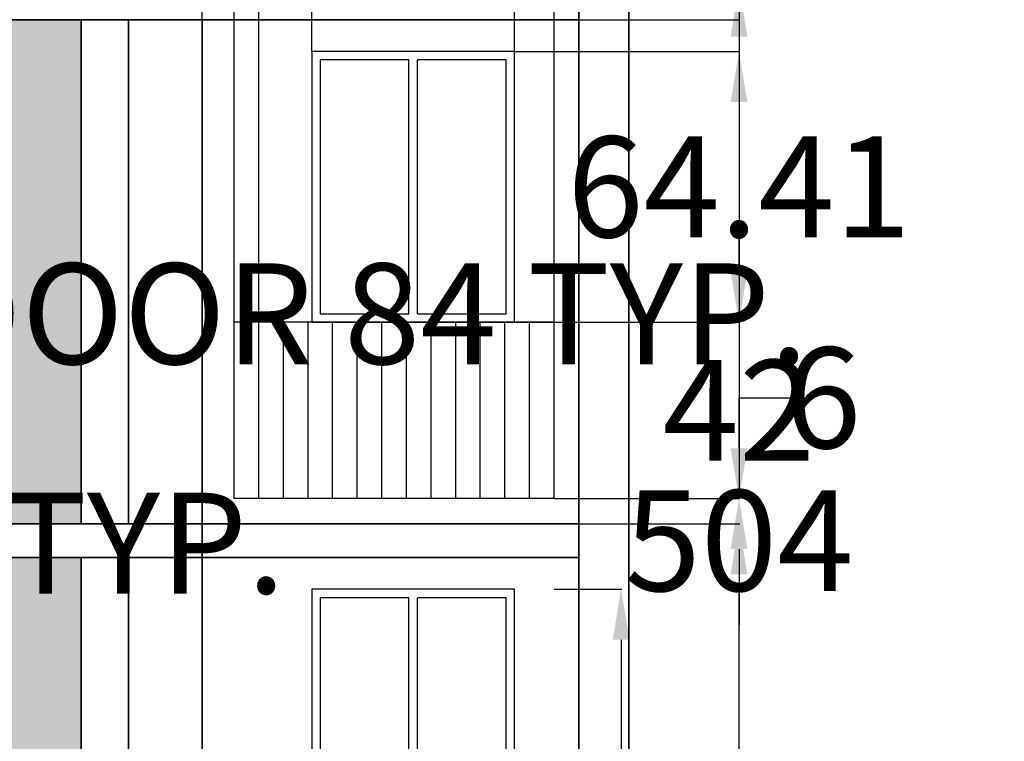
# Model space of a CAD drawing. Units: inches. Extents: x 172 to 828, y 190 to 777.
# Tile 5 of 9: x 474 to 708, y 436 to 607. Entities that reach past the tile are written whole.
import ezdxf

# ---------------------------------------------------------------- set-up
doc = ezdxf.new("R2010")
doc.units = ezdxf.units.IN
doc.header["$MEASUREMENT"] = 0
for name, color, linetype, lineweight in [('A-ANNO-DIMS', 2, 'Continuous', 18), ('A-ELEV', 7, 'Continuous', 35), ('A-ELEV-PATT', 8, 'Continuous', 13), ('A-GLAZ', 3, 'Continuous', 25)]:
    doc.layers.add(name, color=color, linetype=linetype, lineweight=lineweight)
doc.styles.get("Standard").update_dxf_attribs({"font": 'arial.ttf'})
doc.dimstyles.get("Standard").update_dxf_attribs({"dimtxt": 24, "dimasz": 12, "dimexe": 0.18, "dimexo": 0.0625, "dimgap": 0.09, "dimtad": 0, "dimtih": 1, "dimtoh": 1, "dimdec": 0, "dimzin": 0, "dimdsep": 46, "dimlunit": 3, "dimtxsty": 'Standard', "dimcen": 0.09, "dimadec": 0, "dimazin": 0, "dimtfac": 1, "dimtdec": 0, "dimtofl": 0, "dimtmove": 0, "dimatfit": 3, "dimfxl": 1, "dimtolj": 1, "dimtzin": 0, "dimarcsym": 0})
pattern_1 = [(228.012788, (0.72, 1), (-8, -9), [0.134536, -13.319088]), (184.969741, (0.63, 0.9), (12, 1), [0.230868, -22.8559248]), (132.510447, (0.4, 0.88), (10, -11), [0.162788, -16.1160326]), (267.273689, (0.01, 0.63), (1, 20), [0.210238, -20.813558]), (292.833654, (0, 0.42), (-5, 12), [0.206155, -20.4093731]), (357.273689, (0.08, 0.23), (-20, 1), [0.210238, -20.813558]), (37.6942405, (0.29, 0.22), (-13, -10), [0.278029, -27.5248485]), (72.2553284, (0.51, 0.39), (7, 22), [0.262488, -25.9863215]), (121.4295656, (0.59, 0.64), (-8, 13), [0.21095, -20.8840731]), (175.236358, (0.48, 0.82), (11, -1), [0.240832, -11.8007626]), (222.397438, (0.24, 0.84), (-12, -11), [0.311448, -30.833375]), (138.814075, (1, 0.62), (-7, 6), [0.106301, -10.5238448]), (171.4692344, (0.92, 0.69), (13, -2), [0.202237, -20.0215114]), (225, (0.72, 0.72), (-1e-16, -1), [0.141421, -1.2727926]), (203.19859, (0.65, 0.84), (5, 2), [0.076158, -7.5396151]), (291.80141, (0.58, 0.81), (-1, 3), [0.107703, -5.2774618]), (30.963757, (0.62, 0.71), (3, 2), [0.174929, -5.6560229]), (161.56505, (0.77, 0.8), (2, -1), [0.126491, -3.0357867]), (16.38954, (0, 0.81), (10, 3), [0.1772, -17.5428451]), (70.346176, (0.17, 0.86), (-4, -11), [0.148661, -14.7174077]), (293.19859, (0.77, 1), (-2, 5), [0.152315, -7.4634581]), (343.61046, (0.83, 0.86), (-10, 3), [0.1772, -17.5428451]), (339.443955, (0, 0.19), (-5, 2), [0.17088, -8.3731237]), (294.775141, (0.16, 0.13), (-5, 11), [0.143178, -14.1746431]), (66.80141, (0.78, 0), (2, 5), [0.152315, -7.4634581]), (17.354025, (0.84, 0.14), (-13, -4), [0.167631, -16.5954236]), (69.443955, (0.29, 0), (-2, -5), [0.08544, -8.4585637]), (101.309932, (0.72, 0), (-1, 4), [0.05099, -5.0480295]), (165.963757, (0.71, 0.05), (3, -1), [0.206155, -3.9169506]), (186.009006, (0.51, 0.1), (10, 1), [0.19105, -18.9139232]), (303.690068, (0.62, 0.62), (-1, 2), [0.144222, -3.4613293]), (353.1572266, (0.7, 0.5), (17, -2), [0.251794, -24.9275626]), (60.945396, (0.95, 0.47), (-4, -7), [0.102956, -10.1926741]), (90, (1, 0.56), (-1, 1), [0.06, -0.94]), (120.256437, (0.49, 0.13), (4, -7), [0.138924, -13.75352]), (48.012788, (0.42, 0.25), (8, 9), [0.269072, -13.184552]), (0, (0.6, 0.45), (1, 1), [0.26, -0.74]), (325.3048465, (0.86, 0.45), (10, -7), [0.158114, -15.6532743]), (254.054604, (0.99, 0.36), (-1, -4), [0.145602, -7.1345079]), (207.6459754, (0.95, 0.22), (-19, -10), [0.237065, -23.4694742]), (175.426079, (0.74, 0.11), (-13, 1), [0.250799, -24.8290734])]

# ---------------------------------------------------------------- blocks, each defined once
blk = doc.blocks.new('WIN-BALCONY')
for p, q in [((41.59, 44), (41.59, 104.41)), ((43.59, 44), (43.59, 104.41)), ((76.13, 42), (0, 42)), ((0, 0), (0, 42)), ((5.86, 0), (5.86, 42)), ((11.71, 0), (11.71, 42)), ((17.57, 0), (17.57, 42)), ((23.43, 0), (23.43, 42)), ((29.28, 0), (29.28, 42)), ((35.14, 0), (35.14, 42)), ((40.99, 0), (40.99, 42)), ((46.85, 0), (46.85, 42)), ((52.71, 0), (52.71, 42)), ((58.56, 0), (58.56, 42)), ((64.42, 0), (64.42, 42)), ((70.28, 0), (70.28, 42)), ((76.13, 0), (76.13, 42)), ((76.13, 0), (0, 0))]:
    blk.add_line(p, q)
blk.add_lwpolyline([(18.47, 42), (66.72, 42), (66.72, 106.41), (18.47, 106.41)], close=True)
for points in [[(41.59, 104.41), (20.47, 104.41), (20.47, 44), (41.59, 44)], [(43.59, 44), (64.72, 44), (64.72, 104.41), (43.59, 104.41)]]:
    blk.add_lwpolyline(points)
blk = doc.blocks.new('*D4')
at = {"layer": 'A-ANNO-DIMS', "color": 0, "lineweight": -2, "transparency": 16777216}
for p, q in [((601.02, 471.8), (617.1, 471.8)), ((616.92, 459.8), (616.92, 431.1)), ((616.92, 377.39), (616.92, 406.09)), ((601.02, 365.39), (617.1, 365.39))]:
    blk.add_line(p, q, dxfattribs=at)
at = {"layer": 'A-ANNO-DIMS', "color": 0, "transparency": 16777216}
for points in [[(614.92, 459.8), (618.92, 459.8), (616.92, 471.8)], [(614.92, 377.39), (618.92, 377.39), (616.92, 365.39)]]:
    blk.add_solid(points, dxfattribs=at)
at = {"layer": 'Defpoints', "color": 0, "transparency": 16777216}
for p in [(600.96, 471.8), (616.92, 471.8), (600.96, 365.39)]:
    blk.add_point(p, dxfattribs=at)
at = {"layer": 'A-ANNO-DIMS', "color": 0, "transparency": 16777216, "insert": (616.92, 418.6), "char_height": 24, "attachment_point": 5}
blk.add_mtext('\\A1;BALCONY WINDOW 106 TYP.', dxfattribs=at)
blk = doc.blocks.new('*D6')
at = {"layer": 'A-ANNO-DIMS', "color": 0, "lineweight": -2, "transparency": 16777216}
for p, q in [((411.3, 579.39), (424.02, 579.39)), ((423.84, 567.39), (423.84, 549.9)), ((423.84, 507.39), (423.84, 524.88)), ((411.3, 495.39), (424.02, 495.39))]:
    blk.add_line(p, q, dxfattribs=at)
at = {"layer": 'A-ANNO-DIMS', "color": 0, "transparency": 16777216}
for points in [[(421.84, 567.39), (425.84, 567.39), (423.84, 579.39)], [(421.84, 507.39), (425.84, 507.39), (423.84, 495.39)]]:
    blk.add_solid(points, dxfattribs=at)
at = {"layer": 'Defpoints', "color": 0, "transparency": 16777216}
for p in [(411.24, 579.39), (423.84, 579.39), (411.24, 495.39)]:
    blk.add_point(p, dxfattribs=at)
at = {"layer": 'A-ANNO-DIMS', "color": 0, "transparency": 16777216, "insert": (423.84, 537.39), "char_height": 24, "attachment_point": 5}
blk.add_mtext('\\A1;GLAZED DOUBLE DOOR 84 TYP.', dxfattribs=at)
blk = doc.blocks.new('*D7')
at = {"layer": 'A-ANNO-DIMS', "color": 0, "lineweight": -2, "transparency": 16777216}
for p, q in [((374.66, 495.33), (374.66, 482.61)), ((411.24, 495.33), (411.24, 482.61)), ((386.66, 482.79), (399.24, 482.79)), ((411.24, 482.79), (423.24, 482.79))]:
    blk.add_line(p, q, dxfattribs=at)
at = {"layer": 'A-ANNO-DIMS', "color": 0, "transparency": 16777216}
for points in [[(386.66, 484.79), (386.66, 480.79), (374.66, 482.79)], [(399.24, 484.79), (399.24, 480.79), (411.24, 482.79)]]:
    blk.add_solid(points, dxfattribs=at)
at = {"layer": 'Defpoints', "color": 0, "transparency": 16777216}
for p in [(374.66, 495.39), (411.24, 495.39), (411.24, 482.79)]:
    blk.add_point(p, dxfattribs=at)
at = {"layer": 'A-ANNO-DIMS', "color": 0, "transparency": 16777216, "insert": (481.73, 482.79), "char_height": 24, "attachment_point": 5}
blk.add_mtext('\\A1;37 TYP.', dxfattribs=at)
blk = doc.blocks.new('*D10')
at = {"layer": 'A-ANNO-DIMS', "color": 0, "lineweight": -2, "transparency": 16777216}
for p, q in [((258.78, 231.45), (258.78, 761.27)), ((270.78, 761.09), (412.23, 761.09)), ((606.78, 761.09), (465.33, 761.09)), ((618.78, 735.45), (618.78, 761.27))]:
    blk.add_line(p, q, dxfattribs=at)
at = {"layer": 'A-ANNO-DIMS', "color": 0, "transparency": 16777216}
for points in [[(270.78, 763.09), (270.78, 759.09), (258.78, 761.09)], [(606.78, 763.09), (606.78, 759.09), (618.78, 761.09)]]:
    blk.add_solid(points, dxfattribs=at)
at = {"layer": 'Defpoints', "color": 0, "transparency": 16777216}
for p in [(618.78, 761.09), (618.78, 735.39), (258.78, 231.39)]:
    blk.add_point(p, dxfattribs=at)
at = {"layer": 'A-ANNO-DIMS', "color": 0, "transparency": 16777216, "insert": (438.78, 761.09), "char_height": 24, "attachment_point": 5}
blk.add_mtext('\\A1;360', dxfattribs=at)
blk = doc.blocks.new('*D11')
at = {"layer": 'A-ANNO-DIMS', "color": 0, "lineweight": -2, "transparency": 16777216}
for p, q in [((618.84, 735.39), (645.16, 735.39)), ((644.98, 723.39), (644.98, 495.74)), ((644.98, 243.39), (644.98, 471.05)), ((618.84, 231.39), (645.16, 231.39))]:
    blk.add_line(p, q, dxfattribs=at)
at = {"layer": 'A-ANNO-DIMS', "color": 0, "transparency": 16777216}
for points in [[(642.98, 723.39), (646.98, 723.39), (644.98, 735.39)], [(642.98, 243.39), (646.98, 243.39), (644.98, 231.39)]]:
    blk.add_solid(points, dxfattribs=at)
at = {"layer": 'Defpoints', "color": 0, "transparency": 16777216}
for p in [(618.78, 735.39), (644.98, 735.39), (618.78, 231.39)]:
    blk.add_point(p, dxfattribs=at)
at = {"layer": 'A-ANNO-DIMS', "color": 0, "transparency": 16777216, "insert": (644.98, 483.39), "char_height": 24, "attachment_point": 5}
blk.add_mtext('\\A1;504', dxfattribs=at)
blk = doc.blocks.new('*D64')
at = {"layer": 'A-ANNO-DIMS', "color": 0, "lineweight": -2, "transparency": 16777216}
for p, q in [((644.98, 645.55), (644.98, 657.55)), ((644.98, 657.55), (656.98, 657.55)), ((518.47, 633.55), (645.16, 633.55)), ((518.47, 615.39), (645.16, 615.39)), ((644.98, 603.39), (644.98, 591.39))]:
    blk.add_line(p, q, dxfattribs=at)
at = {"layer": 'A-ANNO-DIMS', "color": 0, "transparency": 16777216}
for points in [[(642.98, 645.55), (646.98, 645.55), (644.98, 633.55)], [(642.98, 603.39), (646.98, 603.39), (644.98, 615.39)]]:
    blk.add_solid(points, dxfattribs=at)
at = {"layer": 'Defpoints', "color": 0, "transparency": 16777216}
for p in [(518.4, 633.55), (644.98, 633.55), (518.4, 615.39)]:
    blk.add_point(p, dxfattribs=at)
at = {"layer": 'A-ANNO-DIMS', "color": 0, "transparency": 16777216, "insert": (696.43, 657.55), "char_height": 24, "attachment_point": 5}
blk.add_mtext('\\A1;18.16', dxfattribs=at)
blk = doc.blocks.new('*D65')
at = {"layer": 'A-ANNO-DIMS', "color": 0, "lineweight": -2, "transparency": 16777216}
for p, q in [((644.98, 633.36), (644.98, 645.36)), ((644.98, 645.36), (656.98, 645.36)), ((527.16, 621.36), (645.16, 621.36)), ((518.47, 615.39), (645.16, 615.39)), ((644.98, 603.39), (644.98, 591.39))]:
    blk.add_line(p, q, dxfattribs=at)
at = {"layer": 'A-ANNO-DIMS', "color": 0, "transparency": 16777216}
for points in [[(642.98, 633.36), (646.98, 633.36), (644.98, 621.36)], [(642.98, 603.39), (646.98, 603.39), (644.98, 615.39)]]:
    blk.add_solid(points, dxfattribs=at)
at = {"layer": 'Defpoints', "color": 0, "transparency": 16777216}
for p in [(527.09, 621.36), (644.98, 621.36), (518.4, 615.39)]:
    blk.add_point(p, dxfattribs=at)
at = {"layer": 'A-ANNO-DIMS', "color": 0, "transparency": 16777216, "insert": (697.55, 645.36), "char_height": 24, "attachment_point": 5}
blk.add_mtext('\\A1;5.966', dxfattribs=at)
blk = doc.blocks.new('*D66')
at = {"layer": 'A-ANNO-DIMS', "color": 0, "lineweight": -2, "transparency": 16777216}
for p, q in [((644.98, 669.37), (644.98, 681.37)), ((568.83, 657.37), (645.16, 657.37)), ((568.83, 621.36), (645.16, 621.36)), ((644.98, 609.36), (644.98, 597.36))]:
    blk.add_line(p, q, dxfattribs=at)
at = {"layer": 'A-ANNO-DIMS', "color": 0, "transparency": 16777216}
for points in [[(642.98, 669.37), (646.98, 669.37), (644.98, 657.37)], [(642.98, 609.36), (646.98, 609.36), (644.98, 621.36)]]:
    blk.add_solid(points, dxfattribs=at)
at = {"layer": 'Defpoints', "color": 0, "transparency": 16777216}
for p in [(568.77, 657.37), (644.98, 657.37), (568.77, 621.36)]:
    blk.add_point(p, dxfattribs=at)
at = {"layer": 'A-ANNO-DIMS', "color": 0, "transparency": 16777216, "insert": (644.98, 639.36), "char_height": 24, "attachment_point": 5}
blk.add_mtext('\\A1;36.01', dxfattribs=at)
blk = doc.blocks.new('*D76')
at = {"layer": 'A-ANNO-DIMS', "color": 0, "lineweight": -2, "transparency": 16777216}
for p, q in [((399.24, 761.09), (387.24, 761.09)), ((411.24, 495.45), (411.24, 761.27)), ((427.59, 495.45), (427.59, 761.27)), ((439.59, 761.09), (451.59, 761.09))]:
    blk.add_line(p, q, dxfattribs=at)
at = {"layer": 'A-ANNO-DIMS', "color": 0, "transparency": 16777216}
for points in [[(399.24, 763.09), (399.24, 759.09), (411.24, 761.09)], [(439.59, 763.09), (439.59, 759.09), (427.59, 761.09)]]:
    blk.add_solid(points, dxfattribs=at)
at = {"layer": 'Defpoints', "color": 0, "transparency": 16777216}
for p in [(427.59, 761.09), (411.24, 495.39), (427.59, 495.39)]:
    blk.add_point(p, dxfattribs=at)
at = {"layer": 'A-ANNO-DIMS', "color": 0, "transparency": 16777216, "insert": (500.36, 761.09), "char_height": 24, "attachment_point": 5}
blk.add_mtext('\\A1;16.356', dxfattribs=at)
blk = doc.blocks.new('*D77')
at = {"layer": 'A-ANNO-DIMS', "color": 0, "lineweight": -2, "transparency": 16777216}
for p, q in [((427.59, 495.45), (427.59, 761.27)), ((439.59, 761.09), (452.34, 761.09)), ((464.34, 495.45), (464.34, 761.27)), ((464.34, 761.09), (476.34, 761.09))]:
    blk.add_line(p, q, dxfattribs=at)
at = {"layer": 'A-ANNO-DIMS', "color": 0, "transparency": 16777216}
for points in [[(439.59, 763.09), (439.59, 759.09), (427.59, 761.09)], [(452.34, 763.09), (452.34, 759.09), (464.34, 761.09)]]:
    blk.add_solid(points, dxfattribs=at)
at = {"layer": 'Defpoints', "color": 0, "transparency": 16777216}
for p in [(464.34, 761.09), (427.59, 495.39), (464.34, 495.39)]:
    blk.add_point(p, dxfattribs=at)
at = {"layer": 'A-ANNO-DIMS', "color": 0, "transparency": 16777216, "insert": (516.86, 761.09), "char_height": 24, "attachment_point": 5}
blk.add_mtext('\\A1;36.74', dxfattribs=at)
blk = doc.blocks.new('*D81')
at = {"layer": 'A-ANNO-DIMS', "color": 0, "lineweight": -2, "transparency": 16777216}
for p, q in [((505.23, 761.09), (493.23, 761.09)), ((517.23, 607.45), (517.23, 761.27)), ((524.83, 493.45), (524.83, 761.27)), ((536.83, 761.09), (548.83, 761.09))]:
    blk.add_line(p, q, dxfattribs=at)
at = {"layer": 'A-ANNO-DIMS', "color": 0, "transparency": 16777216}
for points in [[(505.23, 763.09), (505.23, 759.09), (517.23, 761.09)], [(536.83, 763.09), (536.83, 759.09), (524.83, 761.09)]]:
    blk.add_solid(points, dxfattribs=at)
at = {"layer": 'Defpoints', "color": 0, "transparency": 16777216}
for p in [(524.83, 761.09), (517.23, 607.39), (524.83, 493.39)]:
    blk.add_point(p, dxfattribs=at)
at = {"layer": 'A-ANNO-DIMS', "color": 0, "transparency": 16777216, "insert": (570.66, 761.09), "char_height": 24, "attachment_point": 5}
blk.add_mtext('\\A1;7.6', dxfattribs=at)
blk = doc.blocks.new('*D82')
at = {"layer": 'A-ANNO-DIMS', "color": 0, "lineweight": -2, "transparency": 16777216}
for p, q in [((588.96, 761.09), (576.96, 761.09)), ((600.96, 493.45), (600.96, 761.27)), ((606.82, 607.45), (606.82, 761.27)), ((618.82, 761.09), (630.82, 761.09))]:
    blk.add_line(p, q, dxfattribs=at)
at = {"layer": 'A-ANNO-DIMS', "color": 0, "transparency": 16777216}
for points in [[(588.96, 763.09), (588.96, 759.09), (600.96, 761.09)], [(618.82, 763.09), (618.82, 759.09), (606.82, 761.09)]]:
    blk.add_solid(points, dxfattribs=at)
at = {"layer": 'Defpoints', "color": 0, "transparency": 16777216}
for p in [(606.82, 761.09), (606.82, 607.39), (600.96, 493.39)]:
    blk.add_point(p, dxfattribs=at)
at = {"layer": 'A-ANNO-DIMS', "color": 0, "transparency": 16777216, "insert": (671.39, 761.09), "char_height": 24, "attachment_point": 5}
blk.add_mtext('\\A1;5.856', dxfattribs=at)
blk = doc.blocks.new('*D83')
at = {"layer": 'A-ANNO-DIMS', "color": 0, "lineweight": -2, "transparency": 16777216}
for p, q in [((512.83, 761.09), (500.83, 761.09)), ((524.83, 535.45), (524.83, 761.27)), ((543.3, 599.86), (543.3, 761.27)), ((555.3, 761.09), (567.3, 761.09))]:
    blk.add_line(p, q, dxfattribs=at)
at = {"layer": 'A-ANNO-DIMS', "color": 0, "transparency": 16777216}
for points in [[(512.83, 763.09), (512.83, 759.09), (524.83, 761.09)], [(555.3, 763.09), (555.3, 759.09), (543.3, 761.09)]]:
    blk.add_solid(points, dxfattribs=at)
at = {"layer": 'Defpoints', "color": 0, "transparency": 16777216}
for p in [(543.3, 761.09), (543.3, 599.8), (524.83, 535.39)]:
    blk.add_point(p, dxfattribs=at)
at = {"layer": 'A-ANNO-DIMS', "color": 0, "transparency": 16777216, "insert": (606.75, 761.09), "char_height": 24, "attachment_point": 5}
blk.add_mtext('\\A1;18.47', dxfattribs=at)
blk = doc.blocks.new('*D84')
at = {"layer": 'A-ANNO-DIMS', "color": 0, "lineweight": -2, "transparency": 16777216}
for p, q in [((543.3, 599.86), (543.3, 761.27)), ((555.3, 761.09), (579.54, 761.09)), ((591.54, 599.86), (591.54, 761.27)), ((591.54, 761.09), (603.54, 761.09))]:
    blk.add_line(p, q, dxfattribs=at)
at = {"layer": 'A-ANNO-DIMS', "color": 0, "transparency": 16777216}
for points in [[(555.3, 763.09), (555.3, 759.09), (543.3, 761.09)], [(579.54, 763.09), (579.54, 759.09), (591.54, 761.09)]]:
    blk.add_solid(points, dxfattribs=at)
at = {"layer": 'Defpoints', "color": 0, "transparency": 16777216}
for p in [(591.54, 761.09), (543.3, 599.8), (591.54, 599.8)]:
    blk.add_point(p, dxfattribs=at)
at = {"layer": 'A-ANNO-DIMS', "color": 0, "transparency": 16777216, "insert": (644.7, 761.09), "char_height": 24, "attachment_point": 5}
blk.add_mtext('\\A1;48.25', dxfattribs=at)
blk = doc.blocks.new('*D85')
at = {"layer": 'A-ANNO-DIMS', "color": 0, "lineweight": -2, "transparency": 16777216}
for p, q in [((579.54, 761.09), (567.54, 761.09)), ((591.54, 599.86), (591.54, 761.27)), ((600.96, 535.45), (600.96, 761.27)), ((612.96, 761.09), (624.96, 761.09))]:
    blk.add_line(p, q, dxfattribs=at)
at = {"layer": 'A-ANNO-DIMS', "color": 0, "transparency": 16777216}
for points in [[(579.54, 763.09), (579.54, 759.09), (591.54, 761.09)], [(612.96, 763.09), (612.96, 759.09), (600.96, 761.09)]]:
    blk.add_solid(points, dxfattribs=at)
at = {"layer": 'Defpoints', "color": 0, "transparency": 16777216}
for p in [(600.96, 761.09), (591.54, 599.8), (600.96, 535.39)]:
    blk.add_point(p, dxfattribs=at)
at = {"layer": 'A-ANNO-DIMS', "color": 0, "transparency": 16777216, "insert": (665.63, 761.09), "char_height": 24, "attachment_point": 5}
blk.add_mtext('\\A1;9.415', dxfattribs=at)
blk = doc.blocks.new('*D86')
at = {"layer": 'A-ANNO-DIMS', "color": 0, "lineweight": -2, "transparency": 16777216}
for p, q in [((512.83, 761.09), (500.83, 761.09)), ((524.83, 493.45), (524.83, 761.27)), ((530.68, 493.45), (530.68, 761.27)), ((542.68, 761.09), (554.68, 761.09))]:
    blk.add_line(p, q, dxfattribs=at)
at = {"layer": 'A-ANNO-DIMS', "color": 0, "transparency": 16777216}
for points in [[(512.83, 763.09), (512.83, 759.09), (524.83, 761.09)], [(542.68, 763.09), (542.68, 759.09), (530.68, 761.09)]]:
    blk.add_solid(points, dxfattribs=at)
at = {"layer": 'Defpoints', "color": 0, "transparency": 16777216}
for p in [(530.68, 761.09), (524.83, 493.39), (530.68, 493.39)]:
    blk.add_point(p, dxfattribs=at)
at = {"layer": 'A-ANNO-DIMS', "color": 0, "transparency": 16777216, "insert": (595.26, 761.09), "char_height": 24, "attachment_point": 5}
blk.add_mtext('\\A1;5.856', dxfattribs=at)
blk = doc.blocks.new('*D88')
at = {"layer": 'A-ANNO-DIMS', "color": 0, "lineweight": -2, "transparency": 16777216}
for p, q in [((644.98, 505.39), (644.98, 517.39)), ((644.98, 517.39), (656.98, 517.39)), ((601.02, 493.39), (645.16, 493.39)), ((606.88, 487.39), (645.16, 487.39)), ((644.98, 475.39), (644.98, 463.39))]:
    blk.add_line(p, q, dxfattribs=at)
at = {"layer": 'A-ANNO-DIMS', "color": 0, "transparency": 16777216}
for points in [[(642.98, 505.39), (646.98, 505.39), (644.98, 493.39)], [(642.98, 475.39), (646.98, 475.39), (644.98, 487.39)]]:
    blk.add_solid(points, dxfattribs=at)
at = {"layer": 'Defpoints', "color": 0, "transparency": 16777216}
for p in [(600.96, 493.39), (644.98, 493.39), (606.82, 487.39)]:
    blk.add_point(p, dxfattribs=at)
at = {"layer": 'A-ANNO-DIMS', "color": 0, "transparency": 16777216, "insert": (664.99, 517.39), "char_height": 24, "attachment_point": 5}
blk.add_mtext('\\A1;6', dxfattribs=at)
blk = doc.blocks.new('*D89')
at = {"layer": 'A-ANNO-DIMS', "color": 0, "lineweight": -2, "transparency": 16777216}
for p, q in [((644.979175, 547.392291), (644.979175, 559.392291)), ((601.021944, 535.392291), (645.159175, 535.392291)), ((601.021944, 493.392291), (645.159175, 493.392291)), ((644.979175, 481.392291), (644.979175, 469.392291))]:
    blk.add_line(p, q, dxfattribs=at)
at = {"layer": 'A-ANNO-DIMS', "color": 0, "transparency": 16777216}
for points in [[(642.979175, 547.392291), (646.979175, 547.392291), (644.979175, 535.392291)], [(642.979175, 481.392291), (646.979175, 481.392291), (644.979175, 493.392291)]]:
    blk.add_solid(points, dxfattribs=at)
at = {"layer": 'Defpoints', "color": 0, "transparency": 16777216}
for p in [(600.959444, 535.392291), (644.979175, 535.392291), (600.959444, 493.392291)]:
    blk.add_point(p, dxfattribs=at)
at = {"layer": 'A-ANNO-DIMS', "color": 0, "transparency": 16777216, "insert": (644.979175, 514.392291), "char_height": 24, "attachment_point": 5}
blk.add_mtext('\\A1;42', dxfattribs=at)
blk = doc.blocks.new('*D90')
at = {"layer": 'A-ANNO-DIMS', "color": 0, "lineweight": -2, "transparency": 16777216}
for p, q in [((591.61, 599.8), (645.16, 599.8)), ((644.98, 587.8), (644.98, 579.94)), ((644.98, 547.39), (644.98, 555.25)), ((591.61, 535.39), (645.16, 535.39))]:
    blk.add_line(p, q, dxfattribs=at)
at = {"layer": 'A-ANNO-DIMS', "color": 0, "transparency": 16777216}
for points in [[(642.98, 587.8), (646.98, 587.8), (644.98, 599.8)], [(642.98, 547.39), (646.98, 547.39), (644.98, 535.39)]]:
    blk.add_solid(points, dxfattribs=at)
at = {"layer": 'Defpoints', "color": 0, "transparency": 16777216}
for p in [(591.54, 599.8), (644.98, 599.8), (591.54, 535.39)]:
    blk.add_point(p, dxfattribs=at)
at = {"layer": 'A-ANNO-DIMS', "color": 0, "transparency": 16777216, "insert": (644.98, 567.6), "char_height": 24, "attachment_point": 5}
blk.add_mtext('\\A1;64.41', dxfattribs=at)
blk = doc.blocks.new('*D91')
at = {"layer": 'A-ANNO-DIMS', "color": 0, "lineweight": -2, "transparency": 16777216}
for p, q in [((644.98, 619.39), (644.98, 631.39)), ((644.98, 631.39), (656.98, 631.39)), ((606.88, 607.39), (645.16, 607.39)), ((591.61, 599.8), (645.16, 599.8)), ((644.98, 587.8), (644.98, 575.8))]:
    blk.add_line(p, q, dxfattribs=at)
at = {"layer": 'A-ANNO-DIMS', "color": 0, "transparency": 16777216}
for points in [[(642.98, 619.39), (646.98, 619.39), (644.98, 607.39)], [(642.98, 587.8), (646.98, 587.8), (644.98, 599.8)]]:
    blk.add_solid(points, dxfattribs=at)
at = {"layer": 'Defpoints', "color": 0, "transparency": 16777216}
for p in [(606.82, 607.39), (644.98, 607.39), (591.54, 599.8)]:
    blk.add_point(p, dxfattribs=at)
at = {"layer": 'A-ANNO-DIMS', "color": 0, "transparency": 16777216, "insert": (695.15, 631.39), "char_height": 24, "attachment_point": 5}
blk.add_mtext('\\A1;7.591', dxfattribs=at)

msp = doc.modelspace()

# ---------------------------------------------------------------- hatches: boundary and pattern name
at = {"layer": 'A-ELEV-PATT'}
h = msp.add_hatch(dxfattribs=at)
h.set_pattern_fill('GRAVEL', color=256)
h.set_pattern_definition(pattern_1)
h.paths.add_polyline_path([(438.7792, 351.3923), (414.7792, 351.3923), (414.7792, 249.3923), (438.7792, 249.3923)])
h.paths.add_polyline_path([(480.7792, 351.3923), (456.7792, 351.3923), (456.7792, 249.3923), (480.7792, 249.3923)])
h.paths.add_polyline_path([(488.4232, 479.3923), (472.3356, 479.3923), (472.3356, 359.3923), (488.4232, 359.3923)])
h.paths.add_polyline_path([(488.4232, 607.3923), (472.3356, 607.3923), (472.3356, 487.3923), (488.4232, 487.3923)])
h = msp.add_hatch(dxfattribs=at)
h.set_pattern_fill('GRAVEL', color=256)
h.set_pattern_definition(pattern_1)
h.paths.add_polyline_path([(480.7792, 351.3923), (456.7792, 351.3923), (456.7792, 249.3923), (480.7792, 249.3923)])
h.paths.add_polyline_path([(488.4232, 479.3923), (472.3356, 479.3923), (472.3356, 359.3923), (488.4232, 359.3923)])
h.paths.add_polyline_path([(488.4232, 607.3923), (472.3356, 607.3923), (472.3356, 487.3923), (488.4232, 487.3923)])
h = msp.add_hatch(dxfattribs=at)
h.set_pattern_fill('GRAVEL', color=256, scale=20)
h.set_pattern_definition([(228.01279, (14.4, 20), (-160, -180), [2.69072, -266.38176]), (184.96974, (12.6, 18), (240, 20), [4.61736, -457.1185]), (132.51045, (8, 17.6), (200, -220), [3.25576, -322.32065]), (267.27369, (0.2, 12.6), (20, 400), [4.20476, -416.27116]), (292.83365, (0, 8.4), (-100, 240), [4.1231, -408.18746]), (357.27369, (1.6, 4.6), (-400, 20), [4.20476, -416.27116]), (37.69424, (5.8, 4.4), (-260, -200), [5.56058, -550.49697]), (72.25533, (10.2, 7.8), (140, 440), [5.24976, -519.72643]), (121.42957, (11.8, 12.8), (-160, 260), [4.219, -417.68146]), (175.23636, (9.6, 16.4), (220, -20), [4.81664, -236.01525]), (222.39744, (4.8, 16.8), (-240, -220), [6.22896, -616.6675]), (138.81407, (20, 12.4), (-140, 120), [2.126, -210.4769]), (171.46923, (18.4, 13.8), (260, -40), [4.04474, -400.43023]), (225, (14.4, 14.4), (-2e-15, -20), [2.8284, -25.45585]), (203.1986, (13, 16.8), (100, 40), [1.52316, -150.7923]), (291.8014, (11.6, 16.2), (-20, 60), [2.15406, -105.54924]), (30.96376, (12.4, 14.2), (60, 40), [3.4986, -113.12046]), (161.56505, (15.4, 16), (40, -20), [2.5298, -60.71573]), (16.38954, (0, 16.2), (200, 60), [3.544, -350.8569]), (70.34618, (3.4, 17.2), (-80, -220), [2.97322, -294.34815]), (293.1986, (15.4, 20), (-40, 100), [3.0463, -149.26916]), (343.61046, (16.6, 17.2), (-200, 60), [3.544, -350.8569]), (339.44395, (0, 3.8), (-100, 40), [3.4176, -167.46247]), (294.77514, (3.2, 2.6), (-100, 220), [2.86356, -283.49286]), (66.8014, (15.6, 0), (40, 100), [3.0463, -149.26916]), (17.35402, (16.8, 2.8), (-260, -80), [3.35262, -331.90847]), (69.44395, (5.8, 0), (-40, -100), [1.7088, -169.17127]), (101.30993, (14.4, 0), (-20, 80), [1.0198, -100.9606]), (165.96376, (14.2, 1), (60, -20), [4.1231, -78.339]), (186.009, (10.2, 2), (200, 20), [3.821, -378.27846]), (303.6901, (12.4, 12.4), (-20, 40), [2.88444, -69.2266]), (353.15723, (14, 10), (340, -40), [5.03588, -498.55125]), (60.9454, (19, 9.4), (-80, -140), [2.0591, -203.8535]), (90, (20, 11.2), (-20, 20), [1.2, -18.8]), (120.25644, (9.8, 2.6), (80, -140), [2.77848, -275.0704]), (48.01279, (8.4, 5), (160, 180), [5.38144, -263.69104]), (0, (12, 9), (20, 20), [5.2, -14.8]), (325.30485, (17.2, 9), (200, -140), [3.16228, -313.0655]), (254.0546, (19.8, 7.2), (-20, -80), [2.91204, -142.69016]), (207.64598, (19, 4.4), (-380, -200), [4.7413, -469.38948]), (175.42608, (14.8, 2.2), (-260, 20), [5.01598, -496.58147])])
h.paths.add_polyline_path([(480.7792, 351.3923), (456.7792, 351.3923), (456.7792, 249.3923), (480.7792, 249.3923)])
h.paths.add_polyline_path([(472.3356, 479.3923), (464.3356, 479.3923), (464.3356, 359.3923), (472.3356, 359.3923)])
h.paths.add_polyline_path([(488.4232, 479.3923), (472.3356, 479.3923), (472.3356, 359.3923), (488.4232, 359.3923)])
h.paths.add_polyline_path([(472.3356, 607.3923), (464.3356, 607.3923), (464.3356, 487.3923), (472.3356, 487.3923)])
h.paths.add_polyline_path([(488.4232, 607.3923), (472.3356, 607.3923), (472.3356, 487.3923), (488.4232, 487.3923)])

# ---------------------------------------------------------------- linework, layer by layer
at = {"layer": 'A-ELEV'}
for p, q in [((606.8158, 359.3923), (606.8158, 663.3923)), ((618.7792, 359.3923), (618.7792, 663.3923)), ((606.8158, 607.3923), (258.7792, 607.3923)), ((606.8158, 607.3923), (258.7792, 607.3923)), ((488.4232, 607.3923), (488.4232, 487.3923)), ((499.6941, 607.3923), (499.6941, 487.3923)), ((517.2267, 607.3923), (517.2267, 479.3923)), ((606.8158, 487.3923), (606.8158, 535.3923)), ((606.8158, 487.3923), (258.7792, 487.3923)), ((606.8158, 479.3923), (258.7792, 479.3923)), ((488.4232, 479.3923), (488.4232, 359.3923)), ((499.6941, 479.3923), (499.6941, 359.3923)), ((517.2267, 479.3923), (517.2267, 359.3923))]:
    msp.add_line(p, q, dxfattribs=at)

# ---------------------------------------------------------------- block references
at = {"layer": 'A-GLAZ'}
for p in [(524.827, 493.392), (524.827, 365.392)]:
    msp.add_blockref('WIN-BALCONY', p, dxfattribs=at)

# ---------------------------------------------------------------- dimensions: what is measured, and where the dimension line sits
at = {"layer": 'A-ANNO-DIMS'}
for base, p1, p2, override, picture, middle in [((618.7792, 761.0923), (258.7792, 231.3923), (618.7792, 735.3923), {"dimdec": 0, "dimlfac": 1, "dimrnd": 0, "dimzin": 0, "dimdsep": 46, "dimlunit": 2}, '*D10', (438.7792, 761.0923)), ((427.5926, 761.0923), (411.2362, 495.3923), (427.5926, 495.3923), {"dimdec": 3, "dimlfac": 1, "dimrnd": 0, "dimzin": 0, "dimdsep": 46, "dimlunit": 2}, '*D76', (500.362, 761.0923)), ((464.3356, 761.0923), (427.5926, 495.3923), (464.3356, 495.3923), {"dimdec": 2, "dimlfac": 1, "dimrnd": 0, "dimzin": 0, "dimdsep": 46, "dimlunit": 2}, '*D77', (516.8622, 761.0923)), ((524.8269, 761.0923), (517.2267, 607.3923), (524.8269, 493.3923), {"dimdec": 1, "dimlfac": 1, "dimrnd": 0, "dimzin": 0, "dimdsep": 46, "dimlunit": 2}, '*D81', (570.6577, 761.0923)), ((543.2956, 761.0923), (524.8269, 535.3923), (543.2956, 599.8013), {"dimdec": 2, "dimlfac": 1, "dimrnd": 0, "dimzin": 0, "dimdsep": 46, "dimlunit": 2}, '*D83', (606.7498, 761.0923)), ((530.6832, 761.0923), (524.8269, 493.3923), (530.6832, 493.3923), {"dimdec": 3, "dimlfac": 1, "dimrnd": 0, "dimzin": 0, "dimdsep": 46, "dimlunit": 2}, '*D86', (595.2589, 761.0923)), ((591.5446, 761.0923), (543.2956, 599.8013), (591.5446, 599.8013), {"dimdec": 2, "dimlfac": 1, "dimrnd": 0, "dimzin": 0, "dimdsep": 46, "dimlunit": 2}, '*D84', (644.7014, 761.0923)), ((600.9594, 761.0923), (591.5446, 599.8013), (600.9594, 535.3923), {"dimdec": 3, "dimlfac": 1, "dimrnd": 0, "dimzin": 0, "dimdsep": 46, "dimlunit": 2}, '*D85', (665.6333, 761.0923)), ((606.8158, 761.0923), (600.9594, 493.3923), (606.8158, 607.3923), {"dimdec": 3, "dimlfac": 1, "dimrnd": 0, "dimzin": 0, "dimdsep": 46, "dimlunit": 2}, '*D82', (671.3915, 761.0923))]:
    dim = msp.add_linear_dim(base=base, p1=p1, p2=p2, dimstyle='Standard', override=override, dxfattribs=at)
    dim.commit()
    dim.dimension.update_dxf_attribs({"geometry": picture, "text_midpoint": middle})
for base, p1, p2, override, picture, middle in [((644.9792, 735.3923), (618.7792, 231.3923), (618.7792, 735.3923), {"dimdec": 0, "dimlfac": 1, "dimrnd": 0, "dimzin": 0, "dimdsep": 46, "dimlunit": 2}, '*D11', (644.9792, 483.3923)), ((644.9792, 657.3703), (568.7692, 621.358), (568.7692, 657.3703), {"dimdec": 2, "dimlfac": 1, "dimrnd": 0, "dimzin": 0, "dimdsep": 46, "dimlunit": 2}, '*D66', (644.9792, 639.3642)), ((644.9792, 633.5521), (518.4045, 615.3923), (518.4045, 633.5521), {"dimdec": 2, "dimlfac": 1, "dimrnd": 0, "dimzin": 0, "dimdsep": 46, "dimlunit": 2}, '*D64', (696.4252, 657.5521)), ((644.9792, 621.358), (518.4045, 615.3923), (527.0943, 621.358), {"dimdec": 3, "dimlfac": 1, "dimrnd": 0, "dimzin": 0, "dimdsep": 46, "dimlunit": 2}, '*D65', (697.5549, 645.358)), ((644.9792, 607.3923), (591.5446, 599.8013), (606.8158, 607.3923), {"dimdec": 3, "dimlfac": 1, "dimrnd": 0, "dimzin": 0, "dimdsep": 46, "dimlunit": 2}, '*D91', (695.1483, 631.3923)), ((644.9792, 599.8013), (591.5446, 535.3923), (591.5446, 599.8013), {"dimdec": 2, "dimlfac": 1, "dimrnd": 0, "dimzin": 0, "dimdsep": 46, "dimlunit": 2}, '*D90', (644.9792, 567.5968)), ((644.9792, 535.3923), (600.9594, 493.3923), (600.9594, 535.3923), {"dimdec": 0, "dimlfac": 1, "dimrnd": 0, "dimzin": 0, "dimdsep": 46, "dimlunit": 2}, '*D89', (644.9792, 514.3923)), ((644.9792, 493.3923), (606.8158, 487.3923), (600.9594, 493.3923), {"dimdec": 0, "dimlfac": 1, "dimrnd": 0, "dimzin": 0, "dimdsep": 46, "dimlunit": 2}, '*D88', (664.9928, 517.3923))]:
    dim = msp.add_linear_dim(base=base, p1=p1, p2=p2, angle=90, dimstyle='Standard', override=override, dxfattribs=at)
    dim.commit()
    dim.dimension.update_dxf_attribs({"geometry": picture, "text_midpoint": middle})
for base, p1, p2, text, picture, middle in [((423.8362, 579.3923), (411.2362, 495.3923), (411.2362, 579.3923), 'GLAZED DOUBLE DOOR <> TYP.', '*D6', (423.8362, 537.3923)), ((616.9208, 471.8013), (600.9594, 365.3923), (600.9594, 471.8013), 'BALCONY WINDOW <> TYP.', '*D4', (616.9208, 418.5968))]:
    dim = msp.add_linear_dim(base=base, p1=p1, p2=p2, angle=90, text=text, dimstyle='Standard', override={"dimdec": 0, "dimlfac": 1, "dimrnd": 0, "dimzin": 0, "dimdsep": 46, "dimlunit": 2}, dxfattribs=at)
    dim.commit()
    dim.dimension.update_dxf_attribs({"geometry": picture, "text_midpoint": middle})
dim = msp.add_linear_dim(base=(411.2362, 482.7923), p1=(374.6632, 495.3923), p2=(411.2362, 495.3923), text='<> TYP.', dimstyle='Standard', override={"dimdec": 0, "dimlfac": 1, "dimrnd": 0, "dimzin": 0, "dimdsep": 46, "dimlunit": 2}, dxfattribs=at)
dim.commit()
dim.dimension.update_dxf_attribs({"geometry": '*D7', "text_midpoint": (481.7301, 482.7923)})

doc.saveas('drawing.dxf')
